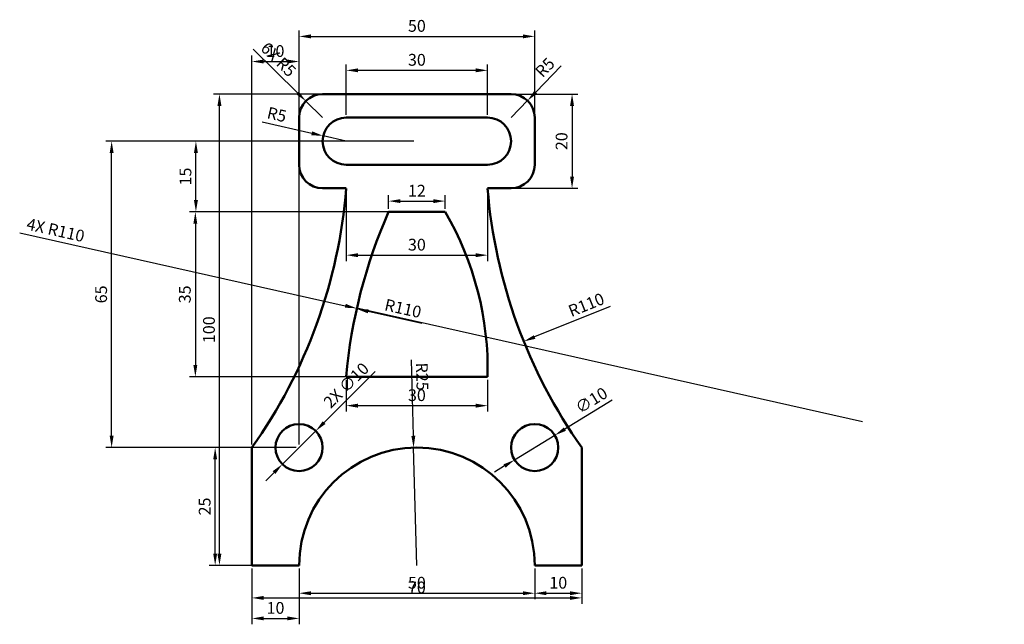
# Model space of a CAD drawing. Units: millimetres. Extents: x 118 to 327, y 39 to 167.
import ezdxf

# ---------------------------------------------------------------- set-up
doc = ezdxf.new("R2010")
doc.units = ezdxf.units.MM
doc.layers.add('M-DIMS', color=2, linetype='Continuous', lineweight=25)
doc.layers.add('M-OUTL', color=7, linetype='Continuous', lineweight=50)
doc.styles.get("Standard").update_dxf_attribs({"font": 'arial.ttf'})
doc.dimstyles.new('ISO-25', dxfattribs={"dimtxt": 2.5, "dimasz": 2.5, "dimexe": 1.25, "dimexo": 0.625, "dimtad": 1, "dimtxsty": 'Standard', "dimcen": 2.5, "dimadec": 0, "dimazin": 0, "dimtfac": 1, "dimtmove": 0, "dimatfit": 3, "dimfxl": 1, "dimarcsym": 0})

# ---------------------------------------------------------------- blocks, each defined once
blk = doc.blocks.new('*D1')
at = {"layer": 'Defpoints', "color": 0, "transparency": 16777216}
for p in [(222.49, 151.44), (222.49, 131.44), (235.42, 131.44)]:
    blk.add_point(p, dxfattribs=at)
at = {"layer": 'M-DIMS', "color": 0, "lineweight": -2, "transparency": 16777216}
for p, q in [((223.12, 151.44), (236.67, 151.44)), ((235.42, 148.94), (235.42, 133.94)), ((223.12, 131.44), (236.67, 131.44))]:
    blk.add_line(p, q, dxfattribs=at)
at = {"layer": 'M-DIMS', "color": 0, "transparency": 16777216}
for points in [[(235, 148.94), (235.83, 148.94), (235.42, 151.44)], [(235, 133.94), (235.83, 133.94), (235.42, 131.44)]]:
    blk.add_solid(points, dxfattribs=at)
at = {"layer": 'M-DIMS', "color": 0, "transparency": 16777216, "insert": (233.52, 141.44), "char_height": 2.5, "attachment_point": 5, "rotation": 90}
blk.add_mtext('20', dxfattribs=at)
blk = doc.blocks.new('*D2')
at = {"layer": 'Defpoints', "color": 0, "transparency": 16777216}
for p in [(225.96, 150.04), (222.49, 146.44)]:
    blk.add_point(p, dxfattribs=at)
at = {"layer": 'M-DIMS', "color": 0, "lineweight": -2, "transparency": 16777216}
for p, q in [((233.11, 157.46), (227.7, 151.84)), ((222.49, 146.44), (225.96, 150.04))]:
    blk.add_line(p, q, dxfattribs=at)
at = {"layer": 'M-DIMS', "color": 0, "transparency": 16777216}
blk.add_solid([(227.4, 152.13), (228, 151.55), (225.96, 150.04)], dxfattribs=at)
at = {"layer": 'M-DIMS', "color": 0, "transparency": 16777216, "insert": (229.9, 156.86), "char_height": 2.5, "attachment_point": 5, "rotation": 46.0613}
blk.add_mtext('R5', dxfattribs=at)
blk = doc.blocks.new('*D3')
at = {"layer": 'Defpoints', "color": 0, "transparency": 16777216}
for p in [(182.62, 142.56), (187.49, 141.44)]:
    blk.add_point(p, dxfattribs=at)
at = {"layer": 'M-DIMS', "color": 0, "lineweight": -2, "transparency": 16777216}
for p, q in [((169.69, 145.53), (180.18, 143.12)), ((187.49, 141.44), (182.62, 142.56))]:
    blk.add_line(p, q, dxfattribs=at)
at = {"layer": 'M-DIMS', "color": 0, "transparency": 16777216}
blk.add_solid([(180.28, 143.53), (180.09, 142.71), (182.62, 142.56)], dxfattribs=at)
at = {"layer": 'M-DIMS', "color": 0, "transparency": 16777216, "insert": (172.7, 146.79), "char_height": 2.5, "attachment_point": 5, "rotation": 347.0398}
blk.add_mtext('R5', dxfattribs=at)
blk = doc.blocks.new('*D4')
at = {"layer": 'Defpoints', "color": 0, "transparency": 16777216}
for p in [(187.49, 156.47), (187.49, 146.44), (217.49, 146.44)]:
    blk.add_point(p, dxfattribs=at)
at = {"layer": 'M-DIMS', "color": 0, "lineweight": -2, "transparency": 16777216}
for p, q in [((187.49, 147.06), (187.49, 157.72)), ((217.49, 147.06), (217.49, 157.72)), ((214.99, 156.47), (189.99, 156.47))]:
    blk.add_line(p, q, dxfattribs=at)
at = {"layer": 'M-DIMS', "color": 0, "transparency": 16777216}
for points in [[(189.99, 156.89), (189.99, 156.06), (187.49, 156.47)], [(214.99, 156.89), (214.99, 156.06), (217.49, 156.47)]]:
    blk.add_solid(points, dxfattribs=at)
at = {"layer": 'M-DIMS', "color": 0, "transparency": 16777216, "insert": (202.49, 158.38), "char_height": 2.5, "attachment_point": 5}
blk.add_mtext('30', dxfattribs=at)
blk = doc.blocks.new('*D5')
at = {"layer": 'Defpoints', "color": 0, "transparency": 16777216}
for p in [(227.49, 163.67), (177.49, 146.44), (227.49, 146.44)]:
    blk.add_point(p, dxfattribs=at)
at = {"layer": 'M-DIMS', "color": 0, "lineweight": -2, "transparency": 16777216}
for p, q in [((177.49, 147.06), (177.49, 164.92)), ((179.99, 163.67), (224.99, 163.67)), ((227.49, 147.06), (227.49, 164.92))]:
    blk.add_line(p, q, dxfattribs=at)
at = {"layer": 'M-DIMS', "color": 0, "transparency": 16777216}
for points in [[(179.99, 164.09), (179.99, 163.26), (177.49, 163.67)], [(224.99, 164.09), (224.99, 163.26), (227.49, 163.67)]]:
    blk.add_solid(points, dxfattribs=at)
at = {"layer": 'M-DIMS', "color": 0, "transparency": 16777216, "insert": (202.49, 165.58), "char_height": 2.5, "attachment_point": 5}
blk.add_mtext('50', dxfattribs=at)
blk = doc.blocks.new('*D6')
at = {"layer": 'Defpoints', "color": 0, "transparency": 16777216}
for p in [(208.49, 128.73), (196.49, 126.44), (208.49, 126.44)]:
    blk.add_point(p, dxfattribs=at)
at = {"layer": 'M-DIMS', "color": 0, "lineweight": -2, "transparency": 16777216}
for p, q in [((196.49, 127.06), (196.49, 129.98)), ((208.49, 127.06), (208.49, 129.98)), ((198.99, 128.73), (205.99, 128.73))]:
    blk.add_line(p, q, dxfattribs=at)
at = {"layer": 'M-DIMS', "color": 0, "transparency": 16777216}
for points in [[(198.99, 129.14), (198.99, 128.31), (196.49, 128.73)], [(205.99, 129.14), (205.99, 128.31), (208.49, 128.73)]]:
    blk.add_solid(points, dxfattribs=at)
at = {"layer": 'M-DIMS', "color": 0, "transparency": 16777216, "insert": (202.49, 130.61), "char_height": 2.5, "attachment_point": 5}
blk.add_mtext('12', dxfattribs=at)
blk = doc.blocks.new('*D7')
at = {"layer": 'Defpoints', "color": 0, "transparency": 16777216}
for p in [(187.49, 91.44), (217.49, 91.44), (217.49, 85.33)]:
    blk.add_point(p, dxfattribs=at)
at = {"layer": 'M-DIMS', "color": 0, "lineweight": -2, "transparency": 16777216}
for p, q in [((187.49, 90.81), (187.49, 84.08)), ((217.49, 90.81), (217.49, 84.08)), ((189.99, 85.33), (214.99, 85.33))]:
    blk.add_line(p, q, dxfattribs=at)
at = {"layer": 'M-DIMS', "color": 0, "transparency": 16777216}
for points in [[(189.99, 85.75), (189.99, 84.91), (187.49, 85.33)], [(214.99, 85.75), (214.99, 84.91), (217.49, 85.33)]]:
    blk.add_solid(points, dxfattribs=at)
at = {"layer": 'M-DIMS', "color": 0, "transparency": 16777216, "insert": (202.49, 87.23), "char_height": 2.5, "attachment_point": 5}
blk.add_mtext('30', dxfattribs=at)
blk = doc.blocks.new('*D8')
at = {"layer": 'Defpoints', "color": 0, "transparency": 16777216}
for p in [(187.49, 131.44), (217.49, 131.44), (217.49, 117.26)]:
    blk.add_point(p, dxfattribs=at)
at = {"layer": 'M-DIMS', "color": 0, "lineweight": -2, "transparency": 16777216}
for p, q in [((187.49, 130.81), (187.49, 116.01)), ((217.49, 130.81), (217.49, 116.01)), ((189.99, 117.26), (214.99, 117.26))]:
    blk.add_line(p, q, dxfattribs=at)
at = {"layer": 'M-DIMS', "color": 0, "transparency": 16777216}
for points in [[(189.99, 117.67), (189.99, 116.84), (187.49, 117.26)], [(214.99, 117.67), (214.99, 116.84), (217.49, 117.26)]]:
    blk.add_solid(points, dxfattribs=at)
at = {"layer": 'M-DIMS', "color": 0, "transparency": 16777216, "insert": (202.49, 119.16), "char_height": 2.5, "attachment_point": 5}
blk.add_mtext('30', dxfattribs=at)
blk = doc.blocks.new('*D9')
at = {"layer": 'Defpoints', "color": 0, "transparency": 16777216}
for p in [(327.14, 140.18), (225.16, 98.96)]:
    blk.add_point(p, dxfattribs=at)
at = {"layer": 'M-DIMS', "color": 0, "lineweight": -2, "transparency": 16777216}
blk.add_line((243.52, 106.38), (227.47, 99.9), dxfattribs=at)
at = {"layer": 'M-DIMS', "color": 0, "transparency": 16777216}
blk.add_solid([(227.32, 100.28), (227.63, 99.51), (225.16, 98.96)], dxfattribs=at)
at = {"layer": 'M-DIMS', "color": 0, "transparency": 16777216, "insert": (238.56, 106.43), "char_height": 2.5, "attachment_point": 5, "rotation": 22.0044}
blk.add_mtext('R110', dxfattribs=at)
blk = doc.blocks.new('*D10')
at = {"layer": 'Defpoints', "color": 0, "transparency": 16777216}
for p in [(189.72, 105.87), (297.08, 81.92)]:
    blk.add_point(p, dxfattribs=at)
at = {"layer": 'M-DIMS', "color": 0, "lineweight": -2, "transparency": 16777216}
blk.add_line((203.54, 102.79), (192.16, 105.32), dxfattribs=at)
at = {"layer": 'M-DIMS', "color": 0, "transparency": 16777216}
blk.add_solid([(192.25, 105.73), (192.07, 104.92), (189.72, 105.87)], dxfattribs=at)
at = {"layer": 'M-DIMS', "color": 0, "transparency": 16777216, "insert": (199.48, 105.64), "char_height": 2.5, "attachment_point": 5, "rotation": 347.4232}
blk.add_mtext('R110', dxfattribs=at)
blk = doc.blocks.new('*D11')
at = {"layer": 'Defpoints', "color": 0, "transparency": 16777216}
for p in [(231.76, 79.05), (223.22, 73.83)]:
    blk.add_point(p, dxfattribs=at)
at = {"layer": 'M-DIMS', "color": 0, "lineweight": -2, "transparency": 16777216}
for p, q in [((243.94, 86.49), (233.89, 80.35)), ((223.22, 73.83), (231.76, 79.05)), ((221.09, 72.53), (218.96, 71.22))]:
    blk.add_line(p, q, dxfattribs=at)
at = {"layer": 'M-DIMS', "color": 0, "transparency": 16777216}
for points in [[(233.67, 80.7), (234.11, 79.99), (231.76, 79.05)], [(220.87, 72.88), (221.31, 72.17), (223.22, 73.83)]]:
    blk.add_solid(points, dxfattribs=at)
at = {"layer": 'M-DIMS', "color": 0, "transparency": 16777216, "insert": (239.69, 86.2), "char_height": 2.5, "attachment_point": 5, "rotation": 31.4276}
blk.add_mtext('∅10', dxfattribs=at)
blk = doc.blocks.new('*D12')
at = {"layer": 'Defpoints', "color": 0, "transparency": 16777216}
for p in [(227.49, 51.44), (237.49, 51.44), (237.49, 45.54)]:
    blk.add_point(p, dxfattribs=at)
at = {"layer": 'M-DIMS', "color": 0, "lineweight": -2, "transparency": 16777216}
for p, q in [((227.49, 50.81), (227.49, 44.29)), ((237.49, 50.81), (237.49, 44.29)), ((229.99, 45.54), (234.99, 45.54))]:
    blk.add_line(p, q, dxfattribs=at)
at = {"layer": 'M-DIMS', "color": 0, "transparency": 16777216}
for points in [[(229.99, 45.95), (229.99, 45.12), (227.49, 45.54)], [(234.99, 45.95), (234.99, 45.12), (237.49, 45.54)]]:
    blk.add_solid(points, dxfattribs=at)
at = {"layer": 'M-DIMS', "color": 0, "transparency": 16777216, "insert": (232.49, 47.44), "char_height": 2.5, "attachment_point": 5}
blk.add_mtext('10', dxfattribs=at)
blk = doc.blocks.new('*D13')
at = {"layer": 'Defpoints', "color": 0, "transparency": 16777216}
for p in [(167.49, 51.44), (177.49, 51.44), (177.49, 40.19)]:
    blk.add_point(p, dxfattribs=at)
at = {"layer": 'M-DIMS', "color": 0, "lineweight": -2, "transparency": 16777216}
for p, q in [((167.49, 50.81), (167.49, 38.94)), ((177.49, 50.81), (177.49, 38.94)), ((169.99, 40.19), (174.99, 40.19))]:
    blk.add_line(p, q, dxfattribs=at)
at = {"layer": 'M-DIMS', "color": 0, "transparency": 16777216}
for points in [[(169.99, 40.61), (169.99, 39.78), (167.49, 40.19)], [(174.99, 40.61), (174.99, 39.78), (177.49, 40.19)]]:
    blk.add_solid(points, dxfattribs=at)
at = {"layer": 'M-DIMS', "color": 0, "transparency": 16777216, "insert": (172.49, 42.1), "char_height": 2.5, "attachment_point": 5}
blk.add_mtext('10', dxfattribs=at)
blk = doc.blocks.new('*D14')
at = {"layer": 'Defpoints', "color": 0, "transparency": 16777216}
for p in [(177.49, 51.44), (227.49, 51.44), (227.49, 45.54)]:
    blk.add_point(p, dxfattribs=at)
at = {"layer": 'M-DIMS', "color": 0, "lineweight": -2, "transparency": 16777216}
for p, q in [((177.49, 50.81), (177.49, 44.29)), ((227.49, 50.81), (227.49, 44.29)), ((179.99, 45.54), (224.99, 45.54))]:
    blk.add_line(p, q, dxfattribs=at)
at = {"layer": 'M-DIMS', "color": 0, "transparency": 16777216}
for points in [[(179.99, 45.95), (179.99, 45.12), (177.49, 45.54)], [(224.99, 45.95), (224.99, 45.12), (227.49, 45.54)]]:
    blk.add_solid(points, dxfattribs=at)
at = {"layer": 'M-DIMS', "color": 0, "transparency": 16777216, "insert": (202.49, 47.44), "char_height": 2.5, "attachment_point": 5}
blk.add_mtext('50', dxfattribs=at)
blk = doc.blocks.new('*D15')
at = {"layer": 'Defpoints', "color": 0, "transparency": 16777216}
for p in [(159.68, 76.44), (177.49, 76.44), (177.49, 51.44)]:
    blk.add_point(p, dxfattribs=at)
at = {"layer": 'M-DIMS', "color": 0, "lineweight": -2, "transparency": 16777216}
for p, q in [((176.87, 76.44), (158.43, 76.44)), ((159.68, 53.94), (159.68, 73.94)), ((176.87, 51.44), (158.43, 51.44))]:
    blk.add_line(p, q, dxfattribs=at)
at = {"layer": 'M-DIMS', "color": 0, "transparency": 16777216}
for points in [[(159.27, 73.94), (160.1, 73.94), (159.68, 76.44)], [(159.27, 53.94), (160.1, 53.94), (159.68, 51.44)]]:
    blk.add_solid(points, dxfattribs=at)
at = {"layer": 'M-DIMS', "color": 0, "transparency": 16777216, "insert": (157.78, 63.94), "char_height": 2.5, "attachment_point": 5, "rotation": 90}
blk.add_mtext('25', dxfattribs=at)
blk = doc.blocks.new('*D16')
at = {"layer": 'Defpoints', "color": 0, "transparency": 16777216}
for p in [(202.49, 126.44), (155.48, 91.44), (202.49, 91.44)]:
    blk.add_point(p, dxfattribs=at)
at = {"layer": 'M-DIMS', "color": 0, "lineweight": -2, "transparency": 16777216}
for p, q in [((201.87, 126.44), (154.23, 126.44)), ((155.48, 123.94), (155.48, 93.94)), ((201.87, 91.44), (154.23, 91.44))]:
    blk.add_line(p, q, dxfattribs=at)
at = {"layer": 'M-DIMS', "color": 0, "transparency": 16777216}
for points in [[(155.06, 123.94), (155.89, 123.94), (155.48, 126.44)], [(155.06, 93.94), (155.89, 93.94), (155.48, 91.44)]]:
    blk.add_solid(points, dxfattribs=at)
at = {"layer": 'M-DIMS', "color": 0, "transparency": 16777216, "insert": (153.57, 108.94), "char_height": 2.5, "attachment_point": 5, "rotation": 90}
blk.add_mtext('35', dxfattribs=at)
blk = doc.blocks.new('*D17')
at = {"layer": 'Defpoints', "color": 0, "transparency": 16777216}
for p in [(155.6, 141.44), (202.49, 141.44), (202.49, 126.44)]:
    blk.add_point(p, dxfattribs=at)
at = {"layer": 'M-DIMS', "color": 0, "lineweight": -2, "transparency": 16777216}
for p, q in [((201.87, 141.44), (154.35, 141.44)), ((155.6, 128.94), (155.6, 138.94)), ((201.87, 126.44), (154.35, 126.44))]:
    blk.add_line(p, q, dxfattribs=at)
at = {"layer": 'M-DIMS', "color": 0, "transparency": 16777216}
for points in [[(155.18, 138.94), (156.02, 138.94), (155.6, 141.44)], [(155.18, 128.94), (156.02, 128.94), (155.6, 126.44)]]:
    blk.add_solid(points, dxfattribs=at)
at = {"layer": 'M-DIMS', "color": 0, "transparency": 16777216, "insert": (153.7, 133.94), "char_height": 2.5, "attachment_point": 5, "rotation": 90}
blk.add_mtext('15', dxfattribs=at)
blk = doc.blocks.new('*D18')
at = {"layer": 'Defpoints', "color": 0, "transparency": 16777216}
for p in [(137.72, 141.44), (177.49, 141.44), (177.49, 76.44)]:
    blk.add_point(p, dxfattribs=at)
at = {"layer": 'M-DIMS', "color": 0, "lineweight": -2, "transparency": 16777216}
for p, q in [((176.87, 141.44), (136.47, 141.44)), ((137.72, 78.94), (137.72, 138.94)), ((176.87, 76.44), (136.47, 76.44))]:
    blk.add_line(p, q, dxfattribs=at)
at = {"layer": 'M-DIMS', "color": 0, "transparency": 16777216}
for points in [[(137.3, 138.94), (138.13, 138.94), (137.72, 141.44)], [(137.3, 78.94), (138.13, 78.94), (137.72, 76.44)]]:
    blk.add_solid(points, dxfattribs=at)
at = {"layer": 'M-DIMS', "color": 0, "transparency": 16777216, "insert": (135.81, 108.94), "char_height": 2.5, "attachment_point": 5, "rotation": 90}
blk.add_mtext('65', dxfattribs=at)
blk = doc.blocks.new('THRU-HOLE-D10')
blk.add_circle((5, 5), 5)
blk = doc.blocks.new('*D20')
at = {"layer": 'Defpoints', "color": 0, "transparency": 16777216}
for p in [(167.49, 51.44), (237.49, 51.44), (237.49, 44.54)]:
    blk.add_point(p, dxfattribs=at)
at = {"layer": 'M-DIMS', "color": 0, "lineweight": -2, "transparency": 16777216}
for p, q in [((167.49, 50.81), (167.49, 43.29)), ((237.49, 50.81), (237.49, 43.29)), ((169.99, 44.54), (234.99, 44.54))]:
    blk.add_line(p, q, dxfattribs=at)
at = {"layer": 'M-DIMS', "color": 0, "transparency": 16777216}
for points in [[(169.99, 44.96), (169.99, 44.12), (167.49, 44.54)], [(234.99, 44.96), (234.99, 44.12), (237.49, 44.54)]]:
    blk.add_solid(points, dxfattribs=at)
at = {"layer": 'M-DIMS', "color": 0, "transparency": 16777216, "insert": (202.49, 46.44), "char_height": 2.5, "attachment_point": 5}
blk.add_mtext('70', dxfattribs=at)
blk = doc.blocks.new('*D21')
at = {"layer": 'Defpoints', "color": 0, "transparency": 16777216}
for p in [(160.59, 151.44), (182.49, 151.44), (167.49, 51.44)]:
    blk.add_point(p, dxfattribs=at)
at = {"layer": 'M-DIMS', "color": 0, "lineweight": -2, "transparency": 16777216}
for p, q in [((181.87, 151.44), (159.34, 151.44)), ((160.59, 53.94), (160.59, 148.94)), ((166.87, 51.44), (159.34, 51.44))]:
    blk.add_line(p, q, dxfattribs=at)
at = {"layer": 'M-DIMS', "color": 0, "transparency": 16777216}
for points in [[(160.17, 148.94), (161.01, 148.94), (160.59, 151.44)], [(160.17, 53.94), (161.01, 53.94), (160.59, 51.44)]]:
    blk.add_solid(points, dxfattribs=at)
at = {"layer": 'M-DIMS', "color": 0, "transparency": 16777216, "insert": (158.69, 101.44), "char_height": 2.5, "attachment_point": 5, "rotation": 90}
blk.add_mtext('100', dxfattribs=at)
blk = doc.blocks.new('*D22')
at = {"layer": 'Defpoints', "color": 0, "transparency": 16777216}
for p in [(177.49, 158.34), (167.49, 76.44), (177.49, 76.44)]:
    blk.add_point(p, dxfattribs=at)
at = {"layer": 'M-DIMS', "color": 0, "lineweight": -2, "transparency": 16777216}
for p, q in [((167.49, 77.06), (167.49, 159.59)), ((177.49, 77.06), (177.49, 159.59)), ((169.99, 158.34), (174.99, 158.34))]:
    blk.add_line(p, q, dxfattribs=at)
at = {"layer": 'M-DIMS', "color": 0, "transparency": 16777216}
for points in [[(169.99, 158.76), (169.99, 157.92), (167.49, 158.34)], [(174.99, 158.76), (174.99, 157.92), (177.49, 158.34)]]:
    blk.add_solid(points, dxfattribs=at)
at = {"layer": 'M-DIMS', "color": 0, "transparency": 16777216, "insert": (172.49, 160.24), "char_height": 2.5, "attachment_point": 5}
blk.add_mtext('10', dxfattribs=at)
blk = doc.blocks.new('*D23')
at = {"layer": 'Defpoints', "color": 0, "transparency": 16777216}
for p in [(201.8, 76.43), (202.49, 51.44)]:
    blk.add_point(p, dxfattribs=at)
at = {"layer": 'M-DIMS', "color": 0, "lineweight": -2, "transparency": 16777216}
for p, q in [((201.28, 95.04), (201.73, 78.93)), ((202.49, 51.44), (201.8, 76.43))]:
    blk.add_line(p, q, dxfattribs=at)
at = {"layer": 'M-DIMS', "color": 0, "transparency": 16777216}
blk.add_solid([(202.15, 78.94), (201.31, 78.92), (201.8, 76.43)], dxfattribs=at)
at = {"layer": 'M-DIMS', "color": 0, "transparency": 16777216, "insert": (203.28, 91.48), "char_height": 2.5, "attachment_point": 5, "rotation": 271.5867}
blk.add_mtext('R25', dxfattribs=at)
blk = doc.blocks.new('*D24')
at = {"layer": 'Defpoints', "color": 0, "transparency": 16777216}
for p in [(178.93, 149.94), (182.49, 146.44)]:
    blk.add_point(p, dxfattribs=at)
at = {"layer": 'M-DIMS', "color": 0, "lineweight": -2, "transparency": 16777216}
for p, q in [((167.74, 160.94), (177.14, 151.7)), ((182.49, 146.44), (178.93, 149.94))]:
    blk.add_line(p, q, dxfattribs=at)
at = {"layer": 'M-DIMS', "color": 0, "transparency": 16777216}
blk.add_solid([(177.44, 151.99), (176.85, 151.4), (178.93, 149.94)], dxfattribs=at)
at = {"layer": 'M-DIMS', "color": 0, "transparency": 16777216, "insert": (172.88, 158.55), "char_height": 2.5, "attachment_point": 5, "rotation": 315.4824}
blk.add_mtext('6X R5', dxfattribs=at)
blk = doc.blocks.new('*D25')
at = {"layer": 'Defpoints', "color": 0, "transparency": 16777216}
for p in [(181.03, 79.97), (173.95, 72.91)]:
    blk.add_point(p, dxfattribs=at)
at = {"layer": 'M-DIMS', "color": 0, "lineweight": -2, "transparency": 16777216}
for p, q in [((193.65, 92.56), (182.8, 81.74)), ((173.95, 72.91), (181.03, 79.97)), ((172.18, 71.14), (170.41, 69.37))]:
    blk.add_line(p, q, dxfattribs=at)
at = {"layer": 'M-DIMS', "color": 0, "transparency": 16777216}
for points in [[(182.51, 82.03), (183.09, 81.44), (181.03, 79.97)], [(171.89, 71.44), (172.48, 70.85), (173.95, 72.91)]]:
    blk.add_solid(points, dxfattribs=at)
at = {"layer": 'M-DIMS', "color": 0, "transparency": 16777216, "insert": (187.72, 89.43), "char_height": 2.5, "attachment_point": 5, "rotation": 44.9423}
blk.add_mtext('2X ∅10', dxfattribs=at)
blk = doc.blocks.new('*D26')
at = {"layer": 'Defpoints', "color": 0, "transparency": 16777216}
for p in [(189.74, 105.98), (297.08, 81.92)]:
    blk.add_point(p, dxfattribs=at)
at = {"layer": 'M-DIMS', "color": 0, "lineweight": -2, "transparency": 16777216}
for p, q in [((118.2, 122.02), (187.3, 106.53)), ((297.08, 81.92), (189.74, 105.98))]:
    blk.add_line(p, q, dxfattribs=at)
at = {"layer": 'M-DIMS', "color": 0, "transparency": 16777216}
blk.add_solid([(187.39, 106.93), (187.21, 106.12), (189.74, 105.98)], dxfattribs=at)
at = {"layer": 'M-DIMS', "color": 0, "transparency": 16777216, "insert": (125.76, 122.27), "char_height": 2.5, "attachment_point": 5, "rotation": 347.3641}
blk.add_mtext('4X R110', dxfattribs=at)

msp = doc.modelspace()

# ---------------------------------------------------------------- linework, layer by layer
at = {"layer": 'M-OUTL'}
for p, q in [((182.491, 151.439), (222.491, 151.439)), ((202.491, 151.439), (182.491, 151.439)), ((177.491, 146.439), (177.491, 141.439)), ((217.491, 146.439), (187.491, 146.439)), ((227.491, 136.439), (227.491, 146.439)), ((177.491, 141.439), (177.491, 136.439)), ((187.491, 136.439), (217.491, 136.439)), ((182.491, 131.439), (187.491, 131.439)), ((217.491, 131.439), (222.491, 131.439)), ((202.491, 126.439), (196.491, 126.439)), ((202.491, 126.439), (208.491, 126.439)), ((217.491, 91.439), (217.491, 94.714)), ((202.491, 91.439), (187.491, 91.439)), ((202.491, 91.439), (217.491, 91.439)), ((167.491, 76.439), (167.491, 51.439)), ((237.491, 51.439), (237.491, 76.439)), ((167.491, 51.439), (177.491, 51.439)), ((227.491, 51.439), (237.491, 51.439))]:
    msp.add_line(p, q, dxfattribs=at)
for centre, radius, start, end in [((182.491, 146.439), 5, 90, 180), ((222.491, 146.439), 5, 0, 90), ((187.491, 141.439), 5, 90, 270), ((217.491, 141.439), 5, 270, 90), ((182.491, 136.439), 5, 180, 270), ((222.491, 136.439), 5, 270, 0), ((77.839, 140.176), 110, 324.58957, 355.44422), ((327.144, 140.176), 110, 184.55578, 215.41043), ((297.078, 81.916), 110, 156.1246, 175.03385), ((151.306, 93.076), 66.206, 358.58237, 30.25918), ((202.491, 51.439), 25, 0, 180)]:
    msp.add_arc(centre, radius, start, end, dxfattribs=at)

# ---------------------------------------------------------------- block references
for p in [(172.491, 71.439), (222.491, 71.439)]:
    msp.add_blockref('THRU-HOLE-D10', p, dxfattribs=at)

# ---------------------------------------------------------------- dimensions: what is measured, and where the dimension line sits
at = {"layer": 'M-DIMS'}
for base, p1, p2, override, picture, middle in [((227.491, 163.675), (177.491, 146.439), (227.491, 146.439), {"dimclrd": 0, "dimclre": 0, "dimclrt": 0}, '*D5', (202.491, 165.576)), ((177.491, 158.339), (167.491, 76.439), (177.491, 76.439), {"dimdec": 0, "dimlfac": 1, "dimrnd": 0, "dimzin": 0, "dimdsep": 46, "dimlunit": 2}, '*D22', (172.491, 160.24)), ((187.491, 156.475), (217.491, 146.439), (187.491, 146.439), {"dimclrd": 0, "dimclre": 0, "dimclrt": 0}, '*D4', (202.491, 158.377)), ((208.491, 128.725), (196.491, 126.439), (208.491, 126.439), {"dimclrd": 0, "dimclre": 0, "dimclrt": 0}, '*D6', (202.491, 130.605)), ((217.491, 117.257), (187.491, 131.439), (217.491, 131.439), {"dimclrd": 0, "dimclre": 0, "dimclrt": 0}, '*D8', (202.491, 119.16)), ((217.491, 85.33), (187.491, 91.439), (217.491, 91.439), {"dimclrd": 0, "dimclre": 0, "dimclrt": 0}, '*D7', (202.491, 87.232)), ((177.491, 40.194), (167.491, 51.439), (177.491, 51.439), {"dimclrd": 0, "dimclre": 0, "dimclrt": 0}, '*D13', (172.491, 42.095)), ((237.491, 44.539), (167.491, 51.439), (237.491, 51.439), {"dimdec": 0, "dimlfac": 1, "dimrnd": 0, "dimzin": 0, "dimdsep": 46, "dimlunit": 2}, '*D20', (202.491, 46.44)), ((227.491, 45.535), (177.491, 51.439), (227.491, 51.439), {"dimclrd": 0, "dimclre": 0, "dimclrt": 0}, '*D14', (202.491, 47.436)), ((237.491, 45.535), (227.491, 51.439), (237.491, 51.439), {"dimclrd": 0, "dimclre": 0, "dimclrt": 0}, '*D12', (232.491, 47.436))]:
    dim = msp.add_linear_dim(base=base, p1=p1, p2=p2, dimstyle='ISO-25', override=override, dxfattribs=at)
    dim.commit()
    dim.dimension.update_dxf_attribs({"geometry": picture, "text_midpoint": middle})
dim = msp.add_radius_dim(center=(182.491, 146.439), mpoint=(178.926, 149.944), text='6X <>', dimstyle='ISO-25', override={"dimdec": 0, "dimlfac": 1, "dimrnd": 0, "dimzin": 0, "dimdsep": 46, "dimlunit": 2}, dxfattribs=at)
dim.commit()
dim.dimension.update_dxf_attribs({"geometry": '*D24', "text_midpoint": (172.885, 158.552)})
dim = msp.add_radius_dim(center=(222.491, 146.439), mpoint=(225.961, 150.039), dimstyle='ISO-25', override={"dimclrd": 0, "dimclre": 0, "dimclrt": 0}, dxfattribs=at)
dim.commit()
dim.dimension.update_dxf_attribs({"geometry": '*D2', "text_midpoint": (229.904, 156.863)})
for base, p1, p2, override, picture, middle in [((160.591, 151.439), (167.491, 51.439), (182.491, 151.439), {"dimdec": 0, "dimlfac": 1, "dimrnd": 0, "dimzin": 0, "dimdsep": 46, "dimlunit": 2}, '*D21', (158.69, 101.439)), ((235.418, 131.439), (222.491, 151.439), (222.491, 131.439), {"dimclrd": 0, "dimclre": 0, "dimclrt": 0}, '*D1', (233.516, 141.439)), ((137.715, 141.439), (177.491, 76.439), (177.491, 141.439), {"dimclrd": 0, "dimclre": 0, "dimclrt": 0}, '*D18', (135.814, 108.939)), ((155.6, 141.439), (202.491, 126.439), (202.491, 141.439), {"dimclrd": 0, "dimclre": 0, "dimclrt": 0}, '*D17', (153.699, 133.939)), ((155.477, 91.439), (202.491, 126.439), (202.491, 91.439), {"dimclrd": 0, "dimclre": 0, "dimclrt": 0}, '*D16', (153.575, 108.939)), ((159.682, 76.439), (177.491, 51.439), (177.491, 76.439), {"dimclrd": 0, "dimclre": 0, "dimclrt": 0}, '*D15', (157.781, 63.939))]:
    dim = msp.add_linear_dim(base=base, p1=p1, p2=p2, angle=90, dimstyle='ISO-25', override=override, dxfattribs=at)
    dim.commit()
    dim.dimension.update_dxf_attribs({"geometry": picture, "text_midpoint": middle})
for center, mpoint, override, picture, middle in [((187.491, 141.439), (182.619, 142.56), {"dimclrd": 0, "dimclre": 0, "dimclrt": 0}, '*D3', (172.277, 144.94)), ((327.144, 140.176), (225.157, 98.961), {"dimclrd": 0, "dimclre": 0, "dimclrt": 0}, '*D9', (239.275, 104.667)), ((297.078, 81.916), (189.718, 105.869), {"dimclrd": 0, "dimclre": 0, "dimclrt": 0}, '*D10', (199.067, 103.783)), ((202.491, 51.439), (201.799, 76.429), {"dimdec": 0, "dimlfac": 1, "dimrnd": 0, "dimzin": 0, "dimdsep": 46, "dimlunit": 2}, '*D23', (201.384, 91.423))]:
    dim = msp.add_radius_dim(center=center, mpoint=mpoint, dimstyle='ISO-25', override=override, dxfattribs=at)
    dim.commit()
    dim.dimension.update_dxf_attribs({"geometry": picture, "text_midpoint": middle, "dimtype": 164})
dim = msp.add_radius_dim(center=(297.078, 81.916), mpoint=(189.743, 105.979), text='4X <>', dimstyle='ISO-25', override={"dimdec": 0, "dimlfac": 1, "dimrnd": 0, "dimzin": 0, "dimdsep": 46, "dimlunit": 2}, dxfattribs=at)
dim.commit()
dim.dimension.update_dxf_attribs({"geometry": '*D26', "text_midpoint": (125.341, 120.417), "dimtype": 164})
dim = msp.add_diameter_dim_2p(p1=(173.952, 72.907), p2=(181.031, 79.971), text='2X <>', dimstyle='ISO-25', override={"dimdec": 0, "dimlfac": 1, "dimrnd": 0, "dimzin": 0, "dimdsep": 46, "dimlunit": 2}, dxfattribs=at)
dim.commit()
dim.dimension.update_dxf_attribs({"geometry": '*D25', "text_midpoint": (189.108, 88.032)})
dim = msp.add_diameter_dim_2p(p1=(223.225, 73.831), p2=(231.758, 79.046), dimstyle='ISO-25', override={"dimclrd": 0, "dimclre": 0, "dimclrt": 0}, dxfattribs=at)
dim.commit()
dim.dimension.update_dxf_attribs({"geometry": '*D11', "text_midpoint": (240.721, 84.522), "dimtype": 163})

doc.saveas('drawing.dxf')
